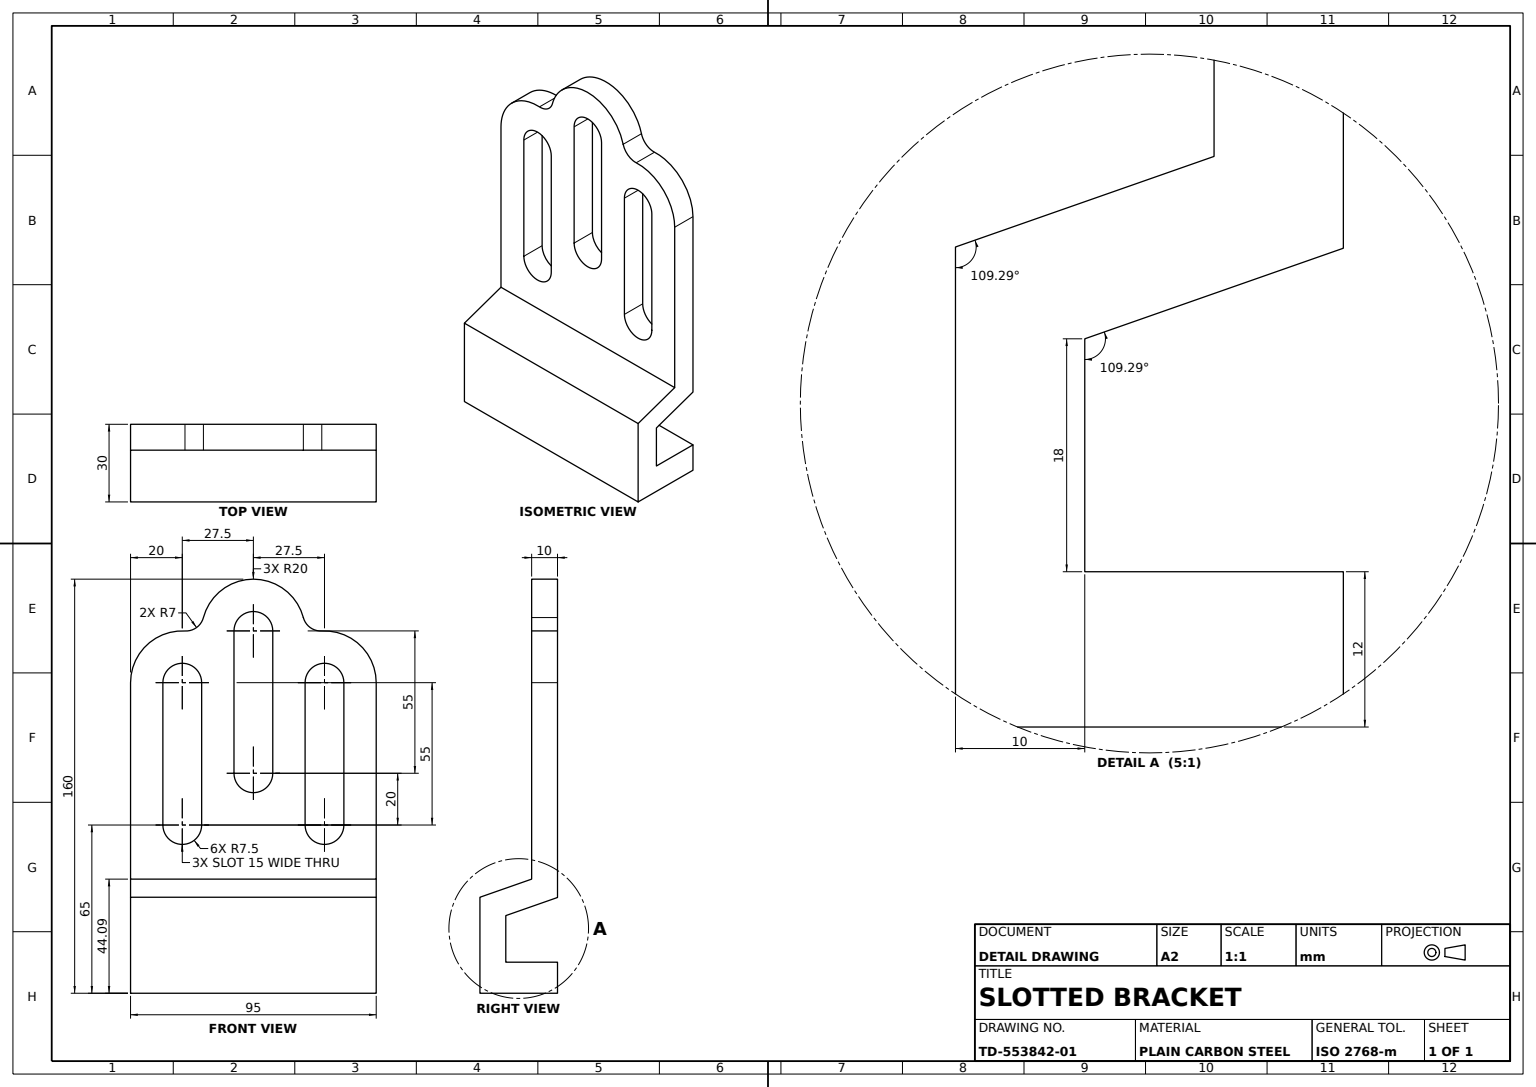
SolidWorks part; units mm, degrees
material "Plain Carbon Steel"
ref_plane "Front Plane" through (0, 0, 0) normal (0, 0, 1) x (1, 0, 0)
ref_plane "Top Plane" through (0, 0, 0) normal (0, 1, 0) x (1, 0, 0)
ref_plane "Right Plane" through (0, 0, 0) normal (1, 0, 0) x (0, 0, -1)
sketch "Support Profile Sketch" plane through (0, 0, 0) normal (0, 0, 1) x (1, 0, 0)
  line L0 (-30, 0) -> (0, 0)
  line L1 (0, 0) -> (0, 37.0948)
  line L2 (0, 37.0948) -> (-20, 44.0948)
  line L3 (-20, 44.0948) -> (-20, 160)
  line L4 (-20, 160) -> (-30, 160)
  line L5 (-30, 160) -> (-30, 37)
  line L6 (-30, 37) -> (-10, 30)
  line L7 (-10, 30) -> (-10, 12)
  line L8 (-10, 12) -> (-30, 12)
  line L9 (-30, 0) -> (-30, 12)
  dimension "D1" = 10
  dimension "D2" = 12
  dimension "D3" = 30
  dimension "D4" = 10
  dimension "D5" = 10
  dimension "D6" = 7
  dimension "D7" = 18
  dimension "D8" = 160
extrude "Support Body" add sketch "Support Profile Sketch" along normal mid plane 95
sketch "Mounting Slots Sketch" plane through (-20, 0, 0) normal (1, 0, 0) x (0, 0, -1)
  line L0 (0, 0) -> (0, 160) construction
  line L1 (-47.5, 160) -> (47.5, 160) construction
  line L2 (-27.5, 120) -> (-27.5, 65) construction
  line L3 (-20, 120) -> (-20, 65)
  line L4 (-35, 120) -> (-35, 65)
  line L5 (27.5, 120) -> (27.5, 65) construction
  line L6 (20, 120) -> (20, 65)
  line L7 (35, 120) -> (35, 65)
  line L8 (47.5, 44.0948) -> (47.5, 160) construction
  line L9 (-47.5, 44.0948) -> (-47.5, 160) construction
  line L10 (47.5, 120) -> (47.5, 160)
  line L11 (-47.5, 160) -> (47.5, 160)
  line L12 (-47.5, 120) -> (-47.5, 160)
  line L13 (0, 140) -> (0, 85) construction
  line L14 (7.5, 140) -> (7.5, 85)
  line L15 (-7.5, 140) -> (-7.5, 85)
  arc A0 (-20, 120) -> (-35, 120) centre (-27.5, 120) ccw
  arc A1 (-35, 65) -> (-20, 65) centre (-27.5, 65) ccw
  arc A2 (20, 120) -> (35, 120) centre (27.5, 120) cw
  arc A3 (35, 65) -> (20, 65) centre (27.5, 65) cw
  arc A5 (-26.4531, 139.9726) -> (-47.5, 120) centre (-27.5, 120) ccw
  arc A6 (26.4531, 139.9726) -> (47.5, 120) centre (27.5, 120) cw
  arc A7 (19.3235, 145.1578) -> (-19.3235, 145.1578) centre (0, 140) ccw
  arc A8 (-19.3235, 145.1578) -> (-26.4531, 139.9726) centre (-26.0867, 146.963) cw
  arc A9 (19.3235, 145.1578) -> (26.4531, 139.9726) centre (26.0867, 146.963) ccw
  arc A10 (7.5, 140) -> (-7.5, 140) centre (0, 140) ccw
  arc A11 (-7.5, 85) -> (7.5, 85) centre (0, 85) ccw
  point P7 (-27.5, 92.5)
  point P15 (27.5, 92.5)
  point P21 (0, 112.5)
  line M22 (47.5, 44.0948) -> (47.5, 160)
  line M23 (47.5, 160) -> (-47.5, 160)
  line M24 (-47.5, 160) -> (-47.5, 44.0948)
  dimension "D5" = 20
  dimension "D6" = 40
  dimension "D7" = 7
  dimension "D8" = 7
  dimension "D3" = 27.5
  dimension "D1" = 40
  dimension "D2" = 55
  dimension "D4" = 15
  dimension "D9" = 55
  dimension "D10" = 15
extrude "Mounting Slots 3x7mm" cut sketch "Mounting Slots Sketch" against normal up to next contours L4 A1 L3 A0 | L15 A11 L14 A10 | A3 L7 A2 L6 | A7 A9 A6 M22 M23 | A8 A7 L11 A5 M24
